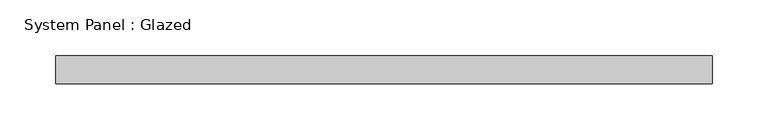
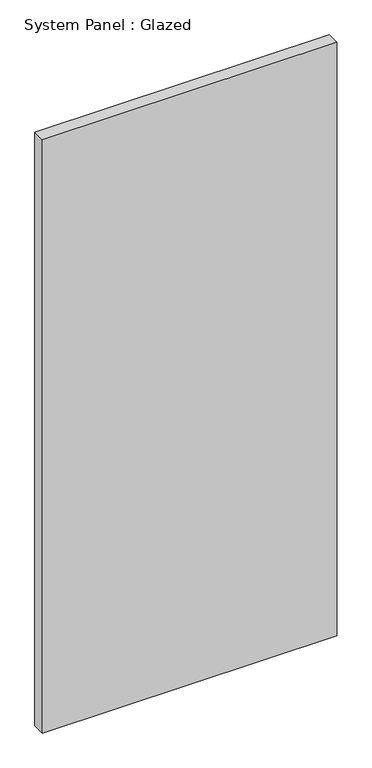
"""IFC4 building model written with IfcOpenShell, lengths in millimetres: plate geometry, System Panel : Glazed."""

from ifc_helpers import new_model, si_unit, origin, origin_with_axes, place, context, project, spatial, polyline, outline, extrude, source, transform, mapped, element, save


def system_panel_glazed_a29d5ab1(model_context):
    return source(origin(), model_context, "Body", "SweptSolid", [
        extrude(outline(polyline([(295.275, 19.05), (-295.275, 19.05), (-295.275, 44.45), (295.275, 44.45), (295.275, 19.05)])), origin_with_axes(), (0.0, 0.0, 1.0), 1257.7839289),
    ])


if __name__ == "__main__":
    model = new_model("IFC4")
    model_context = context("Model", 3, world=origin())
    ifc_project = project(units=[si_unit("LENGTHUNIT", "METRE", prefix="MILLI")], contexts=[model_context])
    site = spatial("IfcSite", under=ifc_project)
    building = spatial("IfcBuilding", under=site)
    placement = place(None, origin())
    system_panel_glazed_shape = system_panel_glazed_a29d5ab1(model_context)
    element("IfcPlate", 1, ObjectType="System Panel : Glazed", at=placement, inside=building, context=model_context, shape_type="MappedRepresentation", body=[
        mapped(system_panel_glazed_shape, transform((0.0, 0.0, 0.0), x_axis=(1.0, 0.0, 0.0), y_axis=(0.0, 1.0, 0.0), z_axis=(0.0, 0.0, 1.0))),
    ])
    save(model, "model.ifc")

# Revit data of these elements
# Type "System Panel : Glazed"
#   Construction Type Id = "GSP4R"
#   Analytic Construction = "1/8 in Pilkington single glazing"
#   Visual Light Transmittance = 0.9
#   Solar Heat Gain Coefficient = 0.86
#   Heat Transfer Coefficient (U) = 1.18115 BTU/(h·ft²·°F)
#   Define Thermal Properties by = 1
# Element 1 (IfcPlate, "System Panel : Glazed")
#   Materials on its faces: "Glass"
# Materials
#   "Glass": class "Glass", colour RGB 0 128 192, transparency 0.75, Description = "Soda Lime Glass", Cost = 0
